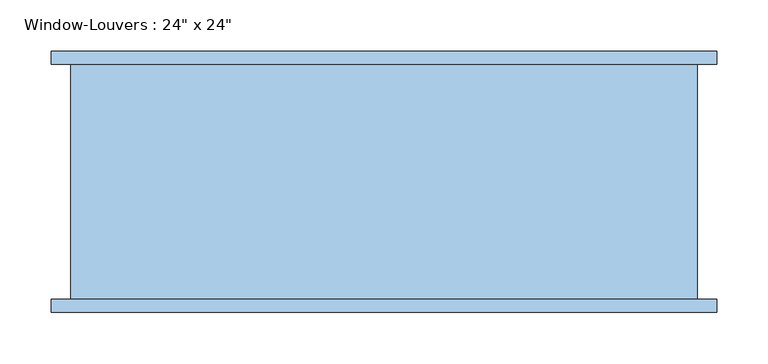
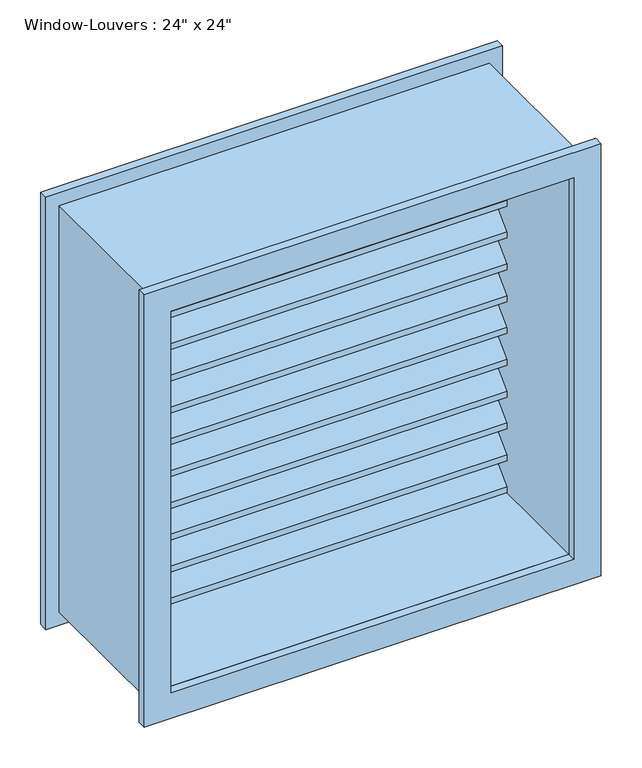
"""IFC4 building model written with IfcOpenShell, lengths in millimetres: window geometry."""

from ifc_helpers import new_model, si_unit, frame, origin, place, context, project, spatial, polyline, outline, extrude, source, transform, mapped, element, save


def window_f2d8fef0(model_context):
    return source(origin(), model_context, "Body", "SweptSolid", [
        extrude(outline(polyline([(107.95, 1419.1754778), (107.95, 1410.1952217), (69.85, 1448.2952217), (31.75, 1410.1952217), (31.75, 1419.1754778), (69.85, 1457.2754778), (107.95, 1419.1754778)])), frame((-285.75, 0.0, 0.0), z_axis=(1.0, 0.0, 0.0), x_axis=(0.0, 1.0, 0.0)), (0.0, 0.0, 1.0), 571.5),
        extrude(outline(polyline([(107.95, 1371.5009557), (107.95, 1362.5206995), (69.85, 1400.6206995), (31.75, 1362.5206995), (31.75, 1371.5009557), (69.85, 1409.6009557), (107.95, 1371.5009557)])), frame((-285.75, 0.0, 0.0), z_axis=(1.0, 0.0, 0.0), x_axis=(0.0, 1.0, 0.0)), (0.0, 0.0, 1.0), 571.5),
        extrude(outline(polyline([(107.95, 1323.8264335), (107.95, 1314.8461774), (69.85, 1352.9461774), (31.75, 1314.8461774), (31.75, 1323.8264335), (69.85, 1361.9264335), (107.95, 1323.8264335)])), frame((-285.75, 0.0, 0.0), z_axis=(1.0, 0.0, 0.0), x_axis=(0.0, 1.0, 0.0)), (0.0, 0.0, 1.0), 571.5),
        extrude(outline(polyline([(107.95, 1276.1519113), (107.95, 1267.1716552), (69.85, 1305.2716552), (31.75, 1267.1716552), (31.75, 1276.1519113), (69.85, 1314.2519113), (107.95, 1276.1519113)])), frame((-285.75, 0.0, 0.0), z_axis=(1.0, 0.0, 0.0), x_axis=(0.0, 1.0, 0.0)), (0.0, 0.0, 1.0), 571.5),
        extrude(outline(polyline([(107.95, 1228.4773891), (107.95, 1219.497133), (69.85, 1257.597133), (31.75, 1219.497133), (31.75, 1228.4773891), (69.85, 1266.5773891), (107.95, 1228.4773891)])), frame((-285.75, 0.0, 0.0), z_axis=(1.0, 0.0, 0.0), x_axis=(0.0, 1.0, 0.0)), (0.0, 0.0, 1.0), 571.5),
        extrude(outline(polyline([(107.95, 1180.802867), (107.95, 1171.8226109), (69.85, 1209.9226109), (31.75, 1171.8226109), (31.75, 1180.802867), (69.85, 1218.902867), (107.95, 1180.802867)])), frame((-285.75, 0.0, 0.0), z_axis=(1.0, 0.0, 0.0), x_axis=(0.0, 1.0, 0.0)), (0.0, 0.0, 1.0), 571.5),
        extrude(outline(polyline([(107.95, 1133.1283448), (107.95, 1124.1480887), (69.85, 1162.2480887), (31.75, 1124.1480887), (31.75, 1133.1283448), (69.85, 1171.2283448), (107.95, 1133.1283448)])), frame((-285.75, 0.0, 0.0), z_axis=(1.0, 0.0, 0.0), x_axis=(0.0, 1.0, 0.0)), (0.0, 0.0, 1.0), 571.5),
        extrude(outline(polyline([(107.95, 1085.4538226), (107.95, 1076.4735665), (69.85, 1114.5735665), (31.75, 1076.4735665), (31.75, 1085.4538226), (69.85, 1123.5538226), (107.95, 1085.4538226)])), frame((-285.75, 0.0, 0.0), z_axis=(1.0, 0.0, 0.0), x_axis=(0.0, 1.0, 0.0)), (0.0, 0.0, 1.0), 571.5),
        extrude(outline(polyline([(107.95, 1037.7793005), (107.95, 1028.7990443), (69.85, 1066.8990443), (31.75, 1028.7990443), (31.75, 1037.7793005), (69.85, 1075.8793005), (107.95, 1037.7793005)])), frame((-285.75, 0.0, 0.0), z_axis=(1.0, 0.0, 0.0), x_axis=(0.0, 1.0, 0.0)), (0.0, 0.0, 1.0), 571.5),
        extrude(outline(polyline([(107.95, 990.1047783), (107.95, 981.1245222), (69.85, 1019.2245222), (31.75, 981.1245222), (31.75, 990.1047783), (69.85, 1028.2047783), (107.95, 990.1047783)])), frame((-285.75, 0.0, 0.0), z_axis=(1.0, 0.0, 0.0), x_axis=(0.0, 1.0, 0.0)), (0.0, 0.0, 1.0), 571.5),
        extrude(outline(polyline([(107.95, 1466.85), (107.95, 1457.8697439), (69.85, 1495.9697439), (31.75, 1457.8697439), (31.75, 1466.85), (69.85, 1504.95), (107.95, 1466.85)])), frame((-285.75, 0.0, 0.0), z_axis=(1.0, 0.0, 0.0), x_axis=(0.0, 1.0, 0.0)), (0.0, 0.0, 1.0), 571.5),
        extrude(outline(polyline([(107.95, 942.4302561), (107.95, 933.45), (69.85, 971.55), (31.75, 933.45), (31.75, 942.4302561), (69.85, 980.5302561), (107.95, 942.4302561)])), frame((-285.75, 0.0, 0.0), z_axis=(1.0, 0.0, 0.0), x_axis=(0.0, 1.0, 0.0)), (0.0, 0.0, 1.0), 571.5),
        extrude(outline(polyline([(1524.0, 304.8), (1524.0, -304.8), (914.4, -304.8), (914.4, 304.8), (1524.0, 304.8)]), holes=[polyline([(1504.95, 285.75), (933.45, 285.75), (933.45, -285.75), (1504.95, -285.75), (1504.95, 285.75)])]), frame((0.0, -120.65, 0.0), z_axis=(0.0, 1.0, 0.0), x_axis=(0.0, 0.0, 1.0)), (0.0, 0.0, 1.0), 228.6),
        extrude(outline(polyline([(1543.05, 323.85), (1543.05, -323.85), (895.35, -323.85), (895.35, 323.85), (1543.05, 323.85)]), holes=[polyline([(1504.95, 285.75), (933.45, 285.75), (933.45, -285.75), (1504.95, -285.75), (1504.95, 285.75)])]), frame((0.0, -133.35, 0.0), z_axis=(0.0, 1.0, 0.0), x_axis=(0.0, 0.0, 1.0)), (0.0, 0.0, 1.0), 12.7),
        extrude(outline(polyline([(1543.05, -323.85), (895.35, -323.85), (895.35, 323.85), (1543.05, 323.85), (1543.05, -323.85)]), holes=[polyline([(1504.95, -285.75), (1504.95, 285.75), (933.45, 285.75), (933.45, -285.75), (1504.95, -285.75)])]), frame((0.0, 107.95, 0.0), z_axis=(0.0, 1.0, 0.0), x_axis=(0.0, 0.0, 1.0)), (0.0, 0.0, 1.0), 12.7),
    ])


if __name__ == "__main__":
    model = new_model("IFC4")
    model_context = context("Model", 3, world=origin())
    ifc_project = project(units=[si_unit("LENGTHUNIT", "METRE", prefix="MILLI")], contexts=[model_context])
    site = spatial("IfcSite", under=ifc_project)
    building = spatial("IfcBuilding", under=site)
    placement = place(None, origin())
    window_shape = window_f2d8fef0(model_context)
    element("IfcWindow", 1, ObjectType="Window-Louvers : 24\" x 24\"", at=placement, inside=building, context=model_context, shape_type="MappedRepresentation", body=[
        mapped(window_shape, transform((0.0, 0.0, 0.0), x_axis=(1.0, 0.0, 0.0), y_axis=(0.0, 1.0, 0.0), z_axis=(0.0, 0.0, 1.0))),
    ])
    save(model, "model.ifc")

# Revit data of these elements
# Type "Window-Louvers : 24\" x 24\""
#   Type Mark = "V"
#   Construction Type Id = "GSP4R"
#   Assembly Code = "B20"
#   Analytic Construction = "1/8 in Pilkington single glazing"
#   Visual Light Transmittance = 0.9
#   Thermal Resistance (R) = 1.53941 (h·ft²·°F)/BTU
#   Solar Heat Gain Coefficient = 0.78
#   Max Height = 1' - 11.74264"
#   Height = 2' - 0"
#   Heat Transfer Coefficient (U) = 0.6496 BTU/(h·ft²·°F)
#   Blade Width [instance default] = 1' - 10 1/2"
#   Blade Vertical Thickness = 0' - 0.35355"
#   Blade Thickness = 0' - 0 1/4"
#   Blade Spacing = 0' - 1 1/2"
#   Blade Height = 0' - 1.85355"
#   Blade Depth = 0' - 3"
#   Blade Angle = 45.00°
#   Default Sill Height = 3' - 0"
#   Trim Projection_Exterior = 0' - 0 1/2"
#   Trim Projection_Interior = 0' - 0 1/2"
#   Trim Width_Exterior = 0' - 1 1/2"
#   Trim Width_Interior = 0' - 1 1/2"
#   Width = 2' - 0"
#   Max Blade Count = 12
#   Define Thermal Properties by = 1
#   Blade Count = 12
#   Frame Material = Birch
#   Louver Material = Birch
#   Trim Exterior Material = Birch
#   Trim Interior Material = Birch
#   Wall Closure = (empty or 0)
# Element 1 (IfcWindow, "Window-Louvers : 24\" x 24\"")
#   Materials on its faces: "Birch"
# Materials
#   "Birch": class "Wood", colour RGB 224 178 126, transparency 0, Description = "Betula Alleghaniensis", Cost = 0
